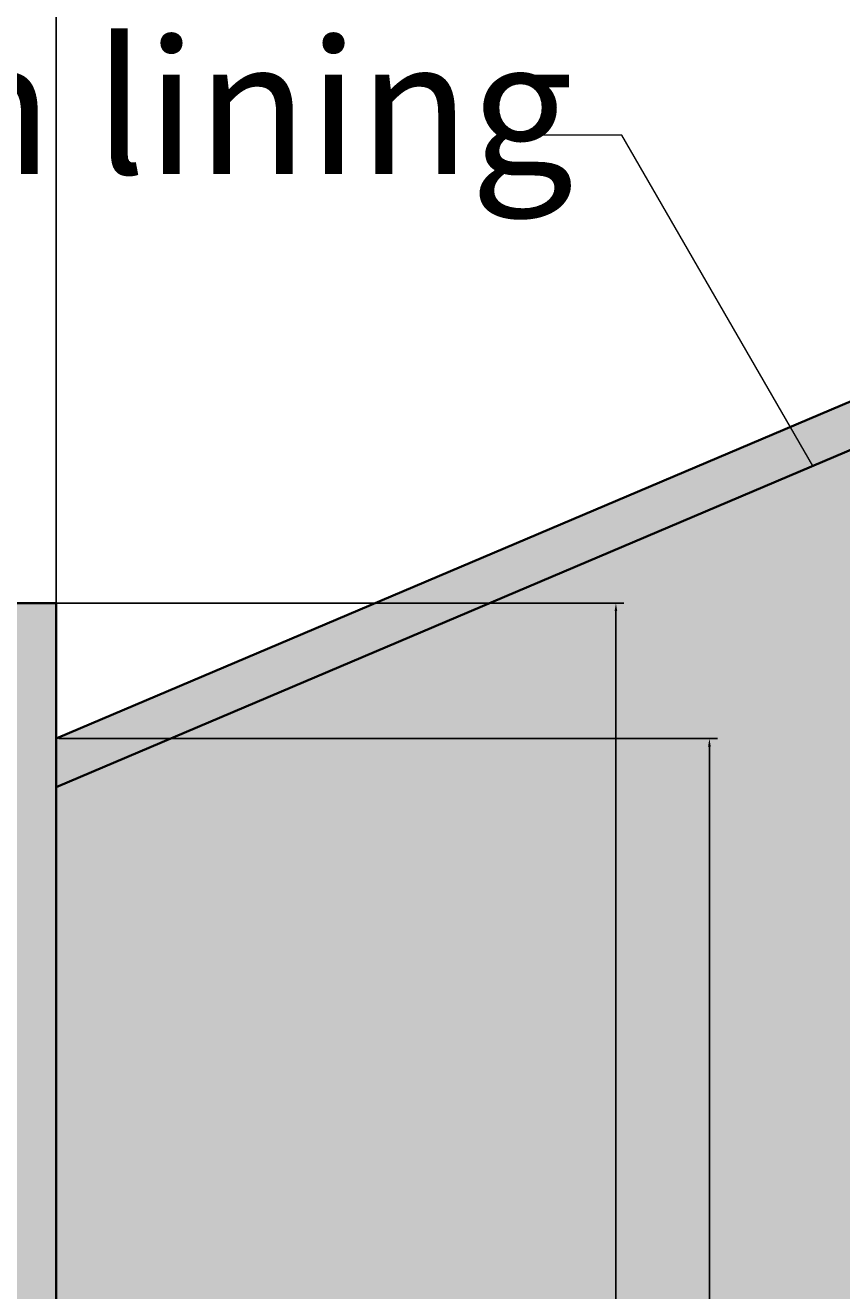
# Model space of a CAD drawing. Units: inches. Extents: x -1 to 292, y -3 to 199.
# Tile 9 of 52: x 23 to 42, y 73 to 101. Entities that reach past the tile are written whole.
import ezdxf

# ---------------------------------------------------------------- set-up
doc = ezdxf.new("R2010")
doc.units = ezdxf.units.IN
doc.header["$MEASUREMENT"] = 0
for name, color, linetype, lineweight in [('M-ANNO-LEAD', 2, 'Continuous', 18), ('M-ANNO-TEXT', 3, 'Continuous', 25), ('M-DIMS', 2, 'Continuous', 18), ('M-EQPM', 7, 'Continuous', 35), ('M-PATT', 8, 'Continuous', 13)]:
    doc.layers.add(name, color=color, linetype=linetype, lineweight=lineweight)
doc.styles.get("Standard").update_dxf_attribs({"font": 'arial.ttf'})
doc.dimstyles.get("Standard").update_dxf_attribs({"dimtxt": 0.18, "dimasz": 0.18, "dimexe": 0.18, "dimexo": 0.0625, "dimgap": 0.09, "dimtad": 0, "dimtih": 1, "dimtoh": 1, "dimdec": 4, "dimzin": 0, "dimdsep": 46, "dimtxsty": 'Standard', "dimcen": 0.09, "dimadec": 0, "dimazin": 0, "dimtfac": 1, "dimtdec": 4, "dimtofl": 0, "dimtmove": 0, "dimatfit": 3, "dimfxl": 1, "dimtolj": 1, "dimtzin": 0, "dimarcsym": 0})

# ---------------------------------------------------------------- blocks, each defined once
blk = doc.blocks.new('DUCT-FLANGE')
for p, q in [((0, 34), (2.089, 34)), ((2.089, 34), (2.089, 0))]:
    blk.add_line(p, q)
blk = doc.blocks.new('*D8')
at = {"layer": 'Defpoints', "color": 0, "transparency": 16777216}
for p in [(-0.662, 126.765), (111.488, 126.765), (69.013, 25.514)]:
    blk.add_point(p, dxfattribs=at)
at = {"layer": 'M-DIMS', "color": 0, "lineweight": -2, "transparency": 16777216}
for p, q in [((111.426, 126.765), (-0.842, 126.765)), ((-0.662, 126.585), (-0.662, 76.321)), ((-0.662, 25.694), (-0.662, 75.958)), ((68.951, 25.514), (-0.842, 25.514))]:
    blk.add_line(p, q, dxfattribs=at)
at = {"layer": 'M-DIMS', "color": 0, "transparency": 16777216}
for points in [[(-0.692, 126.585), (-0.632, 126.585), (-0.662, 126.765)], [(-0.692, 25.694), (-0.632, 25.694), (-0.662, 25.514)]]:
    blk.add_solid(points, dxfattribs=at)
at = {"layer": 'M-DIMS', "color": 0, "transparency": 16777216, "insert": (-0.662, 76.14), "char_height": 0.18, "attachment_point": 5}
blk.add_mtext('\\A1;101.25', dxfattribs=at)
blk = doc.blocks.new('*D14')
at = {"layer": 'Defpoints', "color": 0, "transparency": 16777216}
for p in [(21.861, 88.582), (21.861, 54.582), (36.461, 54.582)]:
    blk.add_point(p, dxfattribs=at)
at = {"layer": 'M-DIMS', "color": 0, "lineweight": -2, "transparency": 16777216}
for p, q in [((21.924, 88.582), (36.641, 88.582)), ((36.461, 88.402), (36.461, 71.764)), ((36.461, 54.762), (36.461, 71.4)), ((21.924, 54.582), (36.641, 54.582))]:
    blk.add_line(p, q, dxfattribs=at)
at = {"layer": 'M-DIMS', "color": 0, "transparency": 16777216}
for points in [[(36.431, 88.402), (36.491, 88.402), (36.461, 88.582)], [(36.431, 54.762), (36.491, 54.762), (36.461, 54.582)]]:
    blk.add_solid(points, dxfattribs=at)
at = {"layer": 'M-DIMS', "color": 0, "transparency": 16777216, "insert": (36.461, 71.582), "char_height": 0.18, "attachment_point": 5}
blk.add_mtext('\\A1;34', dxfattribs=at)
blk = doc.blocks.new('*D15')
at = {"layer": 'Defpoints', "color": 0, "transparency": 16777216}
for p in [(23.95, 174.363), (21.861, 88.582), (23.95, 88.582)]:
    blk.add_point(p, dxfattribs=at)
at = {"layer": 'M-DIMS', "color": 0, "lineweight": -2, "transparency": 16777216}
for p, q in [((21.861, 88.645), (21.861, 174.543)), ((23.95, 88.645), (23.95, 174.543)), ((22.041, 174.363), (22.51, 174.363)), ((23.77, 174.363), (23.301, 174.363))]:
    blk.add_line(p, q, dxfattribs=at)
at = {"layer": 'M-DIMS', "color": 0, "transparency": 16777216}
for points in [[(22.041, 174.393), (22.041, 174.333), (21.861, 174.363)], [(23.77, 174.393), (23.77, 174.333), (23.95, 174.363)]]:
    blk.add_solid(points, dxfattribs=at)
at = {"layer": 'M-DIMS', "color": 0, "transparency": 16777216, "insert": (22.906, 174.363), "char_height": 0.18, "attachment_point": 5}
blk.add_mtext('\\A1;2.089', dxfattribs=at)
blk = doc.blocks.new('*D16')
at = {"layer": 'Defpoints', "color": 0, "transparency": 16777216}
for p in [(42.998, 174.363), (42.998, 93.64), (23.95, 85.555)]:
    blk.add_point(p, dxfattribs=at)
at = {"layer": 'M-DIMS', "color": 0, "lineweight": -2, "transparency": 16777216}
for p, q in [((23.95, 85.618), (23.95, 174.543)), ((42.998, 93.703), (42.998, 174.543)), ((24.13, 174.363), (33.019, 174.363)), ((42.818, 174.363), (33.929, 174.363))]:
    blk.add_line(p, q, dxfattribs=at)
at = {"layer": 'M-DIMS', "color": 0, "transparency": 16777216}
for points in [[(24.13, 174.393), (24.13, 174.333), (23.95, 174.363)], [(42.818, 174.393), (42.818, 174.333), (42.998, 174.363)]]:
    blk.add_solid(points, dxfattribs=at)
at = {"layer": 'M-DIMS', "color": 0, "transparency": 16777216, "insert": (33.474, 174.363), "char_height": 0.18, "attachment_point": 5}
blk.add_mtext('\\A1;19.047', dxfattribs=at)
blk = doc.blocks.new('*D17')
at = {"layer": 'Defpoints', "color": 0, "transparency": 16777216}
for p in [(23.95, 85.555), (23.95, 58.376), (38.55, 58.376)]:
    blk.add_point(p, dxfattribs=at)
at = {"layer": 'M-DIMS', "color": 0, "lineweight": -2, "transparency": 16777216}
for p, q in [((24.013, 85.555), (38.73, 85.555)), ((38.55, 85.375), (38.55, 72.147)), ((38.55, 58.556), (38.55, 71.784)), ((24.013, 58.376), (38.73, 58.376))]:
    blk.add_line(p, q, dxfattribs=at)
at = {"layer": 'M-DIMS', "color": 0, "transparency": 16777216}
for points in [[(38.52, 85.375), (38.58, 85.375), (38.55, 85.555)], [(38.52, 58.556), (38.58, 58.556), (38.55, 58.376)]]:
    blk.add_solid(points, dxfattribs=at)
at = {"layer": 'M-DIMS', "color": 0, "transparency": 16777216, "insert": (38.55, 71.966), "char_height": 0.18, "attachment_point": 5}
blk.add_mtext('\\A1;27.18', dxfattribs=at)

msp = doc.modelspace()

# ---------------------------------------------------------------- hatches: boundary and pattern name
at = {"layer": 'M-PATT'}
h = msp.add_hatch(color=256, dxfattribs=at)
h.set_gradient(color1=(237, 31, 36), color2=(242, 113, 114), tint=1, name='CYLINDER')
h.paths.add_polyline_path([(106.0735, 105.9941), (106.0735, 106.9941), (108.0603, 106.9941), (107.8488, 107.6501), (57.8007, 107.6501, 0.4142136), (49.9241, 99.7735), (52.3176, 101.3278), (55.0097, 99.7735), (57.4032, 101.3278), (60.0953, 99.7735), (62.4888, 101.3278), (65.1809, 99.7735), (67.5744, 101.3278), (70.2665, 99.7735), (72.66, 101.3278), (75.3521, 99.7735), (77.7456, 101.3278), (80.4377, 99.7735), (82.8312, 101.3278), (85.5233, 99.7735), (87.9168, 101.3278), (90.6089, 99.7735), (93.0024, 101.3278), (95.6945, 99.7735), (98.088, 101.3278), (100.7801, 99.7735), (103.1736, 101.3278), (105.8657, 99.7735), (108.2592, 101.3278), (110.9513, 99.7735), (113.3448, 101.3278), (116.0369, 99.7735), (118.4304, 101.3278), (121.1225, 99.7735), (123.516, 101.3278), (126.2082, 99.7735), (128.6016, 101.3278), (131.2938, 99.7735), (133.6872, 101.3278), (136.3794, 99.7735), (138.7728, 101.3278), (141.465, 99.7735), (143.8584, 101.3278), (146.5506, 99.7735), (148.944, 101.3278), (151.6362, 99.7735), (154.0296, 101.3278), (156.7218, 99.7735), (159.1152, 101.3278), (160.6222, 100.4578), (160.6222, 107.6501), (115.4883, 107.6501), (115.4883, 106.9941), (120.9032, 106.9941), (120.9032, 105.9941), (120.9032, 103.3981), (106.0735, 103.3981)])
h.paths.add_polyline_path([(169.176, 107.6501), (162.1623, 107.6501), (162.1623, 100.004), (164.2008, 101.3278), (166.893, 99.7735), (169.2864, 101.3278), (171.9786, 99.7735), (174.372, 101.3278), (177.0526, 99.7802, 0.4139642)])
h.paths.add_polyline_path([(111.4883, 107.6501), (107.8488, 107.6501), (108.0603, 106.9941), (111.4883, 106.9941)], flags=17)
h.paths.add_polyline_path([(61.6788, 91.897), (57.8007, 91.897, -0.1099266), (54.4604, 92.6403), (43.2011, 92.6403), (23.9502, 84.4688), (23.9502, 58.376), (43.2011, 47.2615), (50.9409, 47.2615, -0.2705926), (57.8007, 51.2672), (61.6788, 51.2672)])
h.paths.add_polyline_path([(73.6788, 91.897), (70.6788, 91.897), (70.6788, 51.2672), (73.6788, 51.2672)])
h.paths.add_polyline_path([(79.6788, 91.897), (76.6788, 91.897), (76.6788, 51.2672), (79.6788, 51.2672)])
h.paths.add_polyline_path([(67.6788, 91.897), (64.6788, 91.897), (64.6788, 51.2672), (67.6788, 51.2672)])
h.paths.add_polyline_path([(101.6788, 91.897), (82.6788, 91.897), (82.6788, 51.2672), (101.6788, 51.2672)])
h.paths.add_polyline_path([(107.6788, 91.897), (104.6788, 91.897), (104.6788, 51.2672), (107.6788, 51.2672)])
h.paths.add_polyline_path([(113.6788, 91.897), (110.6788, 91.897), (110.6788, 51.2672), (113.6788, 51.2672)])
h.paths.add_polyline_path([(119.6788, 91.897), (116.6788, 91.897), (116.6788, 51.2672), (119.6788, 51.2672)])
h.paths.add_polyline_path([(141.6788, 91.897), (122.6788, 91.897), (122.6788, 51.2672), (141.6788, 51.2672)])
h.paths.add_polyline_path([(147.6788, 91.897), (144.6788, 91.897), (144.6788, 51.2672), (147.6788, 51.2672)])
h.paths.add_polyline_path([(153.6788, 91.897), (150.6788, 91.897), (150.6788, 51.2672), (153.6788, 51.2672)])
h.paths.add_polyline_path([(159.6788, 91.897), (156.6788, 91.897), (156.6788, 51.2672), (159.6788, 51.2672)])
h.paths.add_polyline_path([(179.5897, 92.6403), (172.5163, 92.6403, -0.1099266), (169.176, 91.897), (162.6788, 91.897), (162.6788, 51.2672), (169.176, 51.2672, -0.2705926), (176.0358, 47.2615), (179.5897, 47.2615)])
h.paths.add_polyline_path([(203.0265, 84.4688), (183.7755, 92.6403), (181.5897, 92.6403), (181.5897, 47.2615), (183.7755, 47.2615), (203.0265, 58.376)])
h.paths.add_polyline_path([(184.4188, 61.52), (200.7224, 61.52), (200.7224, 77.7532), (184.4188, 77.7532)], flags=24)
h = msp.add_hatch(color=256, dxfattribs=at)
h.set_gradient(color1=(76, 38, 47), color2=(76, 38, 47), tint=1, name='CYLINDER')
h.paths.add_polyline_path([(40.8628, 91.6478), (40.3591, 92.5203), (23.9502, 85.5552), (23.9502, 84.4688)])
h.paths.add_polyline_path([(52.8586, 93.6403), (42.9977, 93.6403), (40.3591, 92.5203), (40.8628, 91.6478), (43.2011, 92.6403), (54.4604, 92.6403, -0.0601508)])
h.paths.add_polyline_path([(23.9502, 88.5821), (21.8612, 88.5821), (21.8612, 54.5821), (23.9502, 54.5821)])
h.paths.add_polyline_path([(23.9502, 58.376), (23.9502, 57.2213), (42.9332, 46.2615), (50.4659, 46.2615, -0.0351813), (50.9409, 47.2615), (43.2011, 47.2615)])
h.paths.add_polyline_path([(179.5897, 93.6403), (174.1181, 93.6403, -0.0601508), (172.5163, 92.6403), (179.5897, 92.6403)])
h.paths.add_polyline_path([(183.979, 93.6403), (181.5897, 93.6403), (181.5897, 92.6403), (183.7755, 92.6403), (203.0265, 84.4688), (203.0265, 85.5552)])
h.paths.add_polyline_path([(205.1155, 88.5821), (203.0265, 88.5821), (203.0265, 54.5821), (205.1155, 54.5821)])
h.paths.add_polyline_path([(203.0265, 57.2213), (203.0265, 58.376), (183.7755, 47.2615), (181.5897, 47.2615), (181.5897, 46.2615), (184.0435, 46.2615)])
h.paths.add_polyline_path([(179.5897, 47.2615), (176.0358, 47.2615, -0.0351813), (176.5107, 46.2615), (179.5897, 46.2615)])

# ---------------------------------------------------------------- linework, layer by layer
at = {"layer": 'M-ANNO-LEAD'}
for p, q in [((36.5938, 99.042), (34.2492, 99.042)), ((40.8628, 91.6478), (36.5938, 99.042))]:
    msp.add_line(p, q, dxfattribs=at)
at = {"layer": 'M-EQPM'}
for points in [[(23.9502, 85.5552), (42.9977, 93.6403), (52.8586, 93.6403)], [(23.9502, 84.4688), (43.2011, 92.6403), (54.4604, 92.6403)]]:
    msp.add_lwpolyline(points, dxfattribs=at)

# ---------------------------------------------------------------- block references
msp.add_blockref('DUCT-FLANGE', (21.861, 54.582), dxfattribs=at)

# ---------------------------------------------------------------- texts
at = {"layer": 'M-ANNO-TEXT', "insert": (5.0709, 101.1707), "char_height": 3, "attachment_point": 1}
msp.add_mtext_dynamic_manual_height_columns('refraction lining', width=47.899539, gutter_width=1, heights=[0], dxfattribs=at)

# ---------------------------------------------------------------- dimensions: what is measured, and where the dimension line sits
at = {"layer": 'M-DIMS'}
for base, p1, p2, picture, middle in [((23.9502, 174.3627), (21.8612, 88.5821), (23.9502, 88.5821), '*D15', (22.9057, 174.3627)), ((42.99769, 174.3627), (23.95023, 85.55517), (42.99769, 93.64034), '*D16', (33.47396, 174.3627))]:
    dim = msp.add_linear_dim(base=base, p1=p1, p2=p2, dimstyle='Standard', override={"dimdec": 3, "dimlfac": 1, "dimrnd": 0, "dimzin": 0, "dimdsep": 46, "dimlunit": 2}, dxfattribs=at)
    dim.commit()
    dim.dimension.update_dxf_attribs({"geometry": picture, "text_midpoint": middle})
for base, p1, p2, angle, override, picture, middle in [((-0.6625, 126.765), (69.013, 25.5141), (111.4883, 126.765), 90, {"dimdec": 2, "dimlfac": 1, "dimrnd": 0, "dimzin": 0, "dimdsep": 46, "dimlunit": 2}, '*D8', (-0.6625, 76.1396)), ((36.4612, 54.5821), (21.8612, 88.5821), (21.8612, 54.5821), 270, {"dimdec": 0, "dimlfac": 1, "dimrnd": 0, "dimzin": 0, "dimdsep": 46, "dimlunit": 2}, '*D14', (36.4612, 71.5821)), ((38.5502, 58.376), (23.9502, 85.5552), (23.9502, 58.376), 270, {"dimdec": 2, "dimlfac": 1, "dimrnd": 0, "dimzin": 0, "dimdsep": 46, "dimlunit": 2}, '*D17', (38.5502, 71.9656))]:
    dim = msp.add_linear_dim(base=base, p1=p1, p2=p2, angle=angle, dimstyle='Standard', override=override, dxfattribs=at)
    dim.commit()
    dim.dimension.update_dxf_attribs({"geometry": picture, "text_midpoint": middle})

doc.saveas('drawing.dxf')
